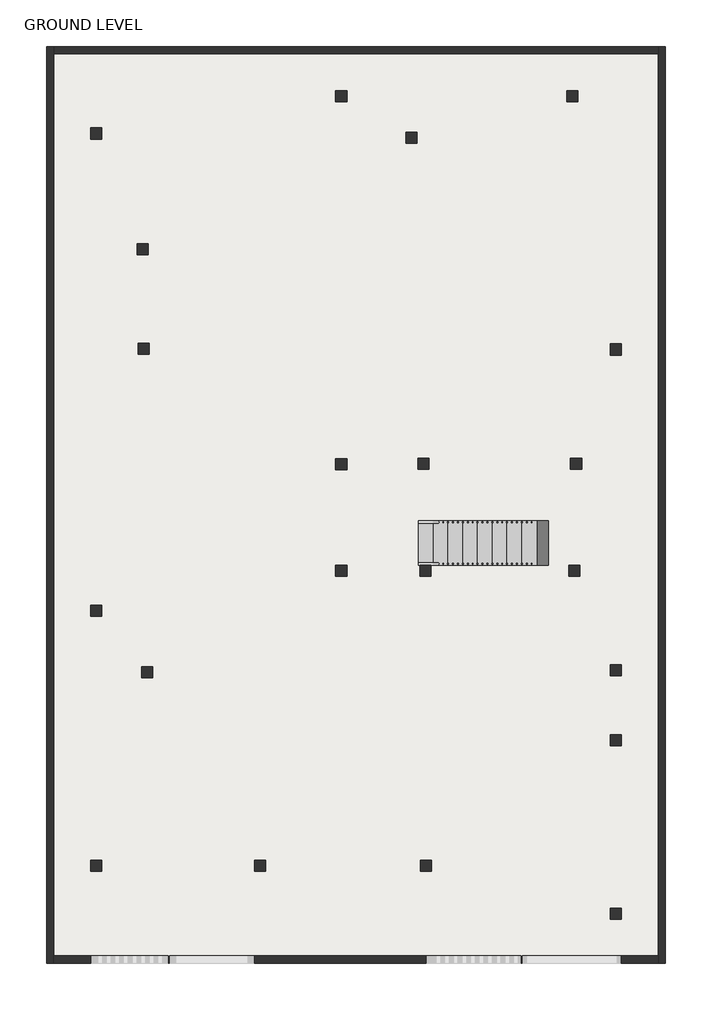
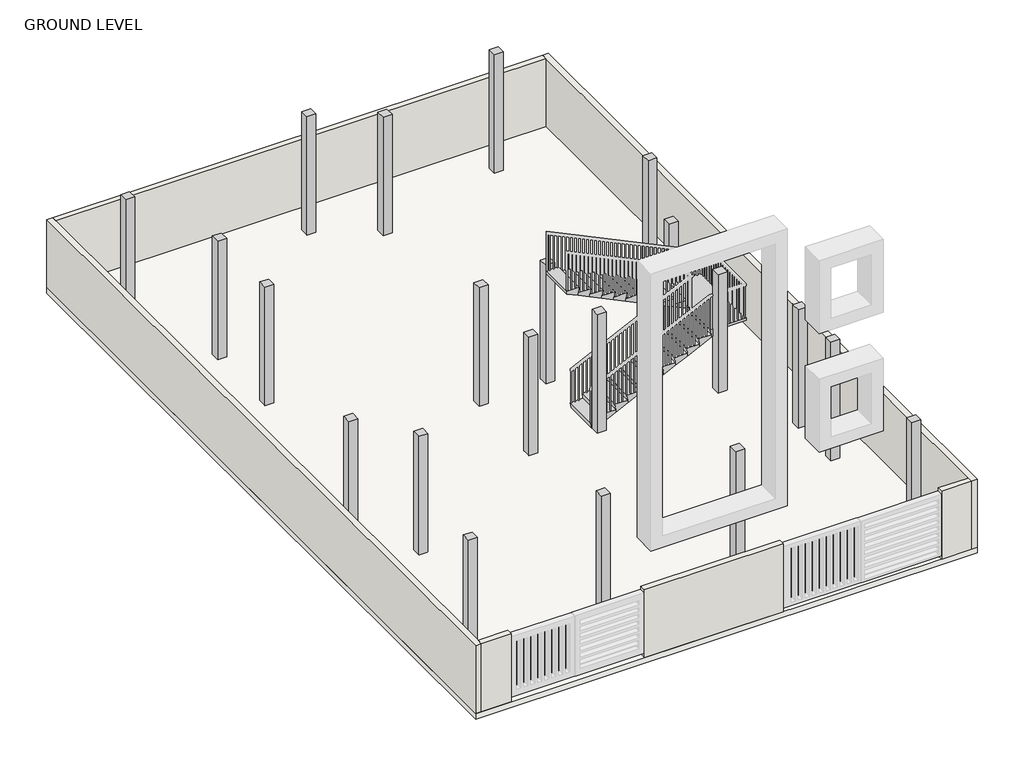
# One storey, part 1 of 3: 21 columns, 6 walls, 1 slab, 1 stair flight.
"""IFC4 building model written with IfcOpenShell, lengths in millimetres."""

from ifc_helpers import new_model, si_unit, frame, origin, origin_with_axes, place, context, project, spatial, polyline, outline, extrude, faceted_brep, element, save

model = new_model("IFC4")

# Units and contexts
model_context = context("Model", 3, world=origin())
ifc_project = project(units=[si_unit("LENGTHUNIT", "METRE", prefix="MILLI")], contexts=[model_context])

# Site, building, storey
site = spatial("IfcSite", under=ifc_project)
building = spatial("IfcBuilding", under=site)
storey = spatial("IfcBuildingStorey", under=building, Name="GROUND LEVEL", Elevation=0.0)

# Columns
placement = place(None, origin())
element("IfcColumn", 1, ObjectType="Rectangular Column : 9\"X9\"", at=placement, inside=storey, context=model_context, shape_type="SweptSolid", body=[
    extrude(outline(polyline([(-6539.8865981, 8531.2343988), (-6539.8865981, 8302.6343988), (-6768.4865981, 8302.6343988), (-6768.4865981, 8531.2343988), (-6539.8865981, 8531.2343988)])), origin_with_axes(), (0.0, 0.0, 1.0), 3200.4),
])
element("IfcColumn", 2, ObjectType="Rectangular Column : 9\"X9\"", at=placement, inside=storey, context=model_context, shape_type="SweptSolid", body=[
    extrude(outline(polyline([(-5558.0284021, 4080.4787587), (-5558.0284021, 3851.8787587), (-5786.6284021, 3851.8787587), (-5786.6284021, 4080.4787587), (-5558.0284021, 4080.4787587)])), origin_with_axes(), (0.0, 0.0, 1.0), 3200.4),
])
element("IfcColumn", 3, ObjectType="Rectangular Column : 9\"X9\"", at=placement, inside=storey, context=model_context, shape_type="SweptSolid", body=[
    extrude(outline(polyline([(-5488.7582398, -2599.7212413), (-5488.7582398, -2828.3212413), (-5717.3582398, -2828.3212413), (-5717.3582398, -2599.7212413), (-5488.7582398, -2599.7212413)])), origin_with_axes(), (0.0, 0.0, 1.0), 3200.4),
])
element("IfcColumn", 4, ObjectType="Rectangular Column : 9\"X9\"", at=placement, inside=storey, context=model_context, shape_type="SweptSolid", body=[
    extrude(outline(polyline([(-6539.8865981, -6601.1424416), (-6539.8865981, -6829.7424416), (-6768.4865981, -6829.7424416), (-6768.4865981, -6601.1424416), (-6539.8865981, -6601.1424416)])), origin_with_axes(), (0.0, 0.0, 1.0), 3200.4),
])
element("IfcColumn", 5, ObjectType="Rectangular Column : 9\"X9\"", at=placement, inside=storey, context=model_context, shape_type="SweptSolid", body=[
    extrude(outline(polyline([(-3148.9865981, -6600.2212413), (-3148.9865981, -6828.8212413), (-3377.5865981, -6828.8212413), (-3377.5865981, -6600.2212413), (-3148.9865981, -6600.2212413)])), origin_with_axes(), (0.0, 0.0, 1.0), 3200.4),
])
element("IfcColumn", 6, ObjectType="Rectangular Column : 9\"X9\"", at=placement, inside=storey, context=model_context, shape_type="SweptSolid", body=[
    extrude(outline(polyline([(280.0134019, -6601.1424416), (280.0134019, -6829.7424416), (51.4134019, -6829.7424416), (51.4134019, -6601.1424416), (280.0134019, -6601.1424416)])), origin_with_axes(), (0.0, 0.0, 1.0), 3200.4),
])
element("IfcColumn", 7, ObjectType="Rectangular Column : 9\"X9\"", at=placement, inside=storey, context=model_context, shape_type="SweptSolid", body=[
    extrude(outline(polyline([(4204.3134019, -7590.8212413), (4204.3134019, -7819.4212413), (3975.7134019, -7819.4212413), (3975.7134019, -7590.8212413), (4204.3134019, -7590.8212413)])), origin_with_axes(), (0.0, 0.0, 1.0), 3200.4),
])
element("IfcColumn", 8, ObjectType="Rectangular Column : 9\"X9\"", at=placement, inside=storey, context=model_context, shape_type="SweptSolid", body=[
    extrude(outline(polyline([(4204.3134019, -4009.4212413), (4204.3134019, -4238.0212413), (3975.7134019, -4238.0212413), (3975.7134019, -4009.4212413), (4204.3134019, -4009.4212413)])), origin_with_axes(), (0.0, 0.0, 1.0), 3200.4),
])
element("IfcColumn", 9, ObjectType="Rectangular Column : 9\"X9\"", at=placement, inside=storey, context=model_context, shape_type="SweptSolid", body=[
    extrude(outline(polyline([(3352.7127672, -504.2212413), (3352.7127672, -732.8212413), (3124.1127672, -732.8212413), (3124.1127672, -504.2212413), (3352.7127672, -504.2212413)])), origin_with_axes(), (0.0, 0.0, 1.0), 3200.4),
])
element("IfcColumn", 10, ObjectType="Rectangular Column : 9\"X9\"", at=placement, inside=storey, context=model_context, shape_type="SweptSolid", body=[
    extrude(outline(polyline([(269.7035962, -504.2212413), (269.7035962, -732.8212413), (41.1035962, -732.8212413), (41.1035962, -504.2212413), (269.7035962, -504.2212413)])), origin_with_axes(), (0.0, 0.0, 1.0), 3200.4),
])
element("IfcColumn", 11, ObjectType="Rectangular Column : 9\"X9\"", at=placement, inside=storey, context=model_context, shape_type="SweptSolid", body=[
    extrude(outline(polyline([(-1472.5865981, -505.1424416), (-1472.5865981, -733.7424416), (-1701.1865981, -733.7424416), (-1701.1865981, -505.1424416), (-1472.5865981, -505.1424416)])), origin_with_axes(), (0.0, 0.0, 1.0), 3200.4),
])
element("IfcColumn", 12, ObjectType="Rectangular Column : 9\"X9\"", at=placement, inside=storey, context=model_context, shape_type="SweptSolid", body=[
    extrude(outline(polyline([(-1472.5865981, 1693.0966521), (-1472.5865981, 1464.4966521), (-1701.1865981, 1464.4966521), (-1701.1865981, 1693.0966521), (-1472.5865981, 1693.0966521)])), origin_with_axes(), (0.0, 0.0, 1.0), 3200.4),
])
element("IfcColumn", 13, ObjectType="Rectangular Column : 9\"X9\"", at=placement, inside=storey, context=model_context, shape_type="SweptSolid", body=[
    extrude(outline(polyline([(229.251657, 1705.5787587), (229.251657, 1476.9787587), (0.651657, 1476.9787587), (0.651657, 1705.5787587), (229.251657, 1705.5787587)])), origin_with_axes(), (0.0, 0.0, 1.0), 3200.4),
])
element("IfcColumn", 14, ObjectType="Rectangular Column : 9\"X9\"", at=placement, inside=storey, context=model_context, shape_type="SweptSolid", body=[
    extrude(outline(polyline([(3385.1070369, 1705.5787587), (3385.1070369, 1476.9787587), (3156.5070369, 1476.9787587), (3156.5070369, 1705.5787587), (3385.1070369, 1705.5787587)])), origin_with_axes(), (0.0, 0.0, 1.0), 3200.4),
])
element("IfcColumn", 15, ObjectType="Rectangular Column : 9\"X9\"", at=placement, inside=storey, context=model_context, shape_type="SweptSolid", body=[
    extrude(outline(polyline([(4204.3134019, 4067.7787587), (4204.3134019, 3839.1787587), (3975.7134019, 3839.1787587), (3975.7134019, 4067.7787587), (4204.3134019, 4067.7787587)])), origin_with_axes(), (0.0, 0.0, 1.0), 3200.4),
])
element("IfcColumn", 16, ObjectType="Rectangular Column : 9\"X9\"", at=placement, inside=storey, context=model_context, shape_type="SweptSolid", body=[
    extrude(outline(polyline([(3305.8577655, 9300.1787587), (3305.8577655, 9071.5787587), (3077.2577655, 9071.5787587), (3077.2577655, 9300.1787587), (3305.8577655, 9300.1787587)])), origin_with_axes(), (0.0, 0.0, 1.0), 3200.4),
])
element("IfcColumn", 17, ObjectType="Rectangular Column : 9\"X9\"", at=placement, inside=storey, context=model_context, shape_type="SweptSolid", body=[
    extrude(outline(polyline([(-24.7865981, 8443.0921256), (-24.7865981, 8214.4921256), (-253.3865981, 8214.4921256), (-253.3865981, 8443.0921256), (-24.7865981, 8443.0921256)])), origin_with_axes(), (0.0, 0.0, 1.0), 3200.4),
])
element("IfcColumn", 18, ObjectType="Rectangular Column : 9\"X9\"", at=placement, inside=storey, context=model_context, shape_type="SweptSolid", body=[
    extrude(outline(polyline([(-5578.456564, 6137.8787587), (-5578.456564, 5909.2787587), (-5807.056564, 5909.2787587), (-5807.056564, 6137.8787587), (-5578.456564, 6137.8787587)])), origin_with_axes(), (0.0, 0.0, 1.0), 3200.4),
])
element("IfcColumn", 19, ObjectType="Rectangular Column : 9\"X9\"", at=placement, inside=storey, context=model_context, shape_type="SweptSolid", body=[
    extrude(outline(polyline([(-6539.8865981, -1329.7212413), (-6539.8865981, -1558.3212413), (-6768.4865981, -1558.3212413), (-6768.4865981, -1329.7212413), (-6539.8865981, -1329.7212413)])), origin_with_axes(), (0.0, 0.0, 1.0), 3200.4),
])
element("IfcColumn", 20, ObjectType="Rectangular Column : 9\"X9\"", at=placement, inside=storey, context=model_context, shape_type="SweptSolid", body=[
    extrude(outline(polyline([(4204.3134019, -2561.6212413), (4204.3134019, -2790.2212413), (3975.7134019, -2790.2212413), (3975.7134019, -2561.6212413), (4204.3134019, -2561.6212413)])), origin_with_axes(), (0.0, 0.0, 1.0), 3200.4),
])
element("IfcColumn", 21, ObjectType="Rectangular Column : 9\"X9\"", at=placement, inside=storey, context=model_context, shape_type="SweptSolid", body=[
    extrude(outline(polyline([(-1472.5865981, 9300.1787587), (-1472.5865981, 9071.5787587), (-1701.1865981, 9071.5787587), (-1701.1865981, 9300.1787587), (-1472.5865981, 9300.1787587)])), origin_with_axes(), (0.0, 0.0, 1.0), 3200.4),
])

# Slab
element("IfcSlab", 22, ObjectType="6\"", at=placement, inside=storey, context=model_context, shape_type="SweptSolid", body=[
    extrude(outline(polyline([(5118.7134019, 10214.5787587), (5118.7134019, -8733.8212413), (-7682.8865981, -8733.8212413), (-7682.8865981, 10214.5787587), (5118.7134019, 10214.5787587)])), frame((0.0, 0.0, -152.4), z_axis=(0.0, 0.0, 1.0), x_axis=(1.0, 0.0, 0.0)), (0.0, 0.0, 1.0), 152.4),
])

# Stair flight
element("IfcStairFlight", 23, ObjectType="3/4\" Nosing", at=placement, inside=storey, context=model_context, shape_type="Brep", body=[
    faceted_brep([(13.3134019, 410.1787587, 145.4727273), (13.3134019, -504.2212413, 145.4727273), (337.1634019, -504.2212413, 145.4727273), (337.1634019, 410.1787587, 145.4727273), (337.1634019, 410.1787587, 75.1111381), (179.7876839, 410.1787587, 0.0), (32.3634019, 410.1787587, 0.0), (32.3634019, -504.2212413, 0.0), (179.7876839, -504.2212413, 0.0), (337.1634019, -504.2212413, 75.1111381), (318.1134019, 410.1787587, 290.9454545), (318.1134019, -504.2212413, 290.9454545), (641.9634019, -504.2212413, 290.9454545), (641.9634019, 410.1787587, 290.9454545), (641.9634019, 410.1787587, 220.5838654), (641.9634019, -504.2212413, 220.5838654), (622.9134019, 410.1787587, 436.4181818), (622.9134019, -504.2212413, 436.4181818), (946.7634019, -504.2212413, 436.4181818), (946.7634019, 410.1787587, 436.4181818), (946.7634019, 410.1787587, 366.0565927), (946.7634019, -504.2212413, 366.0565927), (927.7134019, 410.1787587, 581.8909091), (927.7134019, -504.2212413, 581.8909091), (1251.5634019, -504.2212413, 581.8909091), (1251.5634019, 410.1787587, 581.8909091), (1251.5634019, 410.1787587, 511.5293199), (1251.5634019, -504.2212413, 511.5293199), (1232.5134019, 410.1787587, 727.3636364), (1232.5134019, -504.2212413, 727.3636364), (1556.3634019, -504.2212413, 727.3636364), (1556.3634019, 410.1787587, 727.3636364), (1556.3634019, 410.1787587, 657.0020472), (1556.3634019, -504.2212413, 657.0020472), (1537.3134019, 410.1787587, 872.8363636), (1537.3134019, -504.2212413, 872.8363636), (1861.1634019, -504.2212413, 872.8363636), (1861.1634019, 410.1787587, 872.8363636), (1861.1634019, 410.1787587, 802.4747745), (1861.1634019, -504.2212413, 802.4747745), (1842.1134019, 410.1787587, 1018.3090909), (1842.1134019, -504.2212413, 1018.3090909), (2165.9634019, -504.2212413, 1018.3090909), (2165.9634019, 410.1787587, 1018.3090909), (2165.9634019, 410.1787587, 947.9475018), (2165.9634019, -504.2212413, 947.9475018), (2146.9134019, 410.1787587, 1163.7818182), (2146.9134019, -504.2212413, 1163.7818182), (2470.7634019, -504.2212413, 1163.7818182), (2470.7634019, 410.1787587, 1163.7818182), (2470.7634019, 410.1787587, 1093.420229), (2470.7634019, -504.2212413, 1093.420229), (2451.7134019, 410.1787587, 1309.2545455), (2451.7134019, -504.2212413, 1309.2545455), (2775.5634019, -504.2212413, 1309.2545455), (2775.5634019, 410.1787587, 1309.2545455), (2775.5634019, 410.1787587, 1238.8929563), (2775.5634019, -504.2212413, 1238.8929563), (3080.3634019, 410.1787587, 1454.7272727), (2756.5134019, 410.1787587, 1454.7272727), (2756.5134019, -504.2212413, 1454.7272727), (3080.3634019, -504.2212413, 1454.7272727), (3069.628878, 410.1787587, 1536.7), (3399.5400648, 410.1787587, 1536.7), (3080.3634019, -504.2212413, 1384.3656836), (3042.2634019, 562.5787587, 1600.2), (3061.3134019, 562.5787587, 1600.2), (3061.3134019, 410.1787587, 1600.2), (3061.3134019, -504.2212413, 1600.2), (3399.5400648, -504.2212413, 1600.2), (3975.7134019, -504.2212413, 1600.2), (3975.7134019, 1476.9787587, 1600.2), (3042.2634019, 1476.9787587, 1600.2), (3042.2634019, 562.5787587, 1536.7), (3061.3134019, 562.5787587, 1536.7), (3061.3134019, 410.1787587, 1536.7), (3399.5400648, -504.2212413, 1536.7), (3975.7134019, -504.2212413, 1536.7), (3975.7134019, 1476.9787587, 1536.7), (3042.2634019, 1476.9787587, 1536.7), (3061.3134019, 562.5787587, 1745.6727273), (3061.3134019, 1476.9787587, 1745.6727273), (3027.8867389, 1476.9787587, 1745.6727273), (2737.4634019, 1476.9787587, 1745.6727273), (2737.4634019, 562.5787587, 1745.6727273), (3027.8867389, 562.5787587, 1745.6727273), (2737.4634019, 562.5787587, 1675.3111381), (3027.8867389, 562.5787587, 1536.7), (3027.8867389, 1476.9787587, 1536.7), (2737.4634019, 1476.9787587, 1675.3111381), (2756.5134019, 562.5787587, 1891.1454545), (2756.5134019, 1476.9787587, 1891.1454545), (2432.6634019, 1476.9787587, 1891.1454545), (2432.6634019, 562.5787587, 1891.1454545), (2432.6634019, 562.5787587, 1820.7838654), (2432.6634019, 1476.9787587, 1820.7838654), (2451.7134019, 562.5787587, 2036.6181818), (2451.7134019, 1476.9787587, 2036.6181818), (2127.8634019, 1476.9787587, 2036.6181818), (2127.8634019, 562.5787587, 2036.6181818), (2127.8634019, 562.5787587, 1966.2565927), (2127.8634019, 1476.9787587, 1966.2565927), (2146.9134019, 562.5787587, 2182.0909091), (2146.9134019, 1476.9787587, 2182.0909091), (1823.0634019, 1476.9787587, 2182.0909091), (1823.0634019, 562.5787587, 2182.0909091), (1823.0634019, 562.5787587, 2111.7293199), (1823.0634019, 1476.9787587, 2111.7293199), (1842.1134019, 562.5787587, 2327.5636364), (1842.1134019, 1476.9787587, 2327.5636364), (1518.2634019, 1476.9787587, 2327.5636364), (1518.2634019, 562.5787587, 2327.5636364), (1518.2634019, 562.5787587, 2257.2020472), (1518.2634019, 1476.9787587, 2257.2020472), (1537.3134019, 562.5787587, 2473.0363636), (1537.3134019, 1476.9787587, 2473.0363636), (1213.4634019, 1476.9787587, 2473.0363636), (1213.4634019, 562.5787587, 2473.0363636), (1213.4634019, 562.5787587, 2402.6747745), (1213.4634019, 1476.9787587, 2402.6747745), (1232.5134019, 562.5787587, 2618.5090909), (1232.5134019, 1476.9787587, 2618.5090909), (908.6634019, 1476.9787587, 2618.5090909), (908.6634019, 562.5787587, 2618.5090909), (908.6634019, 562.5787587, 2548.1475018), (908.6634019, 1476.9787587, 2548.1475018), (927.7134019, 562.5787587, 2763.9818182), (927.7134019, 1476.9787587, 2763.9818182), (603.8634019, 1476.9787587, 2763.9818182), (603.8634019, 562.5787587, 2763.9818182), (603.8634019, 562.5787587, 2693.620229), (603.8634019, 1476.9787587, 2693.620229), (622.9134019, 562.5787587, 2909.4545455), (622.9134019, 1476.9787587, 2909.4545455), (299.0634019, 1476.9787587, 2909.4545455), (299.0634019, 562.5787587, 2909.4545455), (299.0634019, 562.5787587, 2839.0929563), (299.0634019, 1476.9787587, 2839.0929563), (318.1134019, 562.5787587, 3054.9272727), (318.1134019, 1476.9787587, 3054.9272727), (13.3134019, 1476.9787587, 3054.9272727), (13.3134019, 562.5787587, 3054.9272727), (13.3134019, 562.5787587, 2975.4736381), (13.3134019, 1476.9787587, 2975.4736381)], [[[0, 1, 2, 3]], [[0, 3, 4, 5, 6]], [[2, 1, 7, 8, 9]], [[10, 11, 12, 13]], [[10, 13, 14, 4, 3]], [[12, 11, 2, 9, 15]], [[16, 17, 18, 19]], [[16, 19, 20, 14, 13]], [[18, 17, 12, 15, 21]], [[22, 23, 24, 25]], [[22, 25, 26, 20, 19]], [[24, 23, 18, 21, 27]], [[28, 29, 30, 31]], [[28, 31, 32, 26, 25]], [[30, 29, 24, 27, 33]], [[34, 35, 36, 37]], [[34, 37, 38, 32, 31]], [[36, 35, 30, 33, 39]], [[40, 41, 42, 43]], [[40, 43, 44, 38, 37]], [[42, 41, 36, 39, 45]], [[46, 47, 48, 49]], [[46, 49, 50, 44, 43]], [[48, 47, 42, 45, 51]], [[52, 53, 54, 55]], [[52, 55, 56, 50, 49]], [[54, 53, 48, 51, 57]], [[58, 59, 60, 61]], [[58, 62, 63, 56, 55, 59]], [[61, 60, 54, 57, 64]], [[65, 66, 67, 68, 69, 70, 71, 72]], [[66, 65, 73, 74]], [[67, 66, 74, 75]], [[62, 67, 75]], [[68, 61, 64, 76, 77, 70, 69]], [[71, 70, 77, 78]], [[72, 71, 78, 79]], [[80, 81, 82, 83, 84, 85]], [[65, 80, 85, 84, 86, 87, 73]], [[81, 72, 79, 88, 89, 83, 82]], [[90, 91, 92, 93]], [[90, 93, 94, 86, 84]], [[92, 91, 83, 89, 95]], [[96, 97, 98, 99]], [[96, 99, 100, 94, 93]], [[98, 97, 92, 95, 101]], [[102, 103, 104, 105]], [[102, 105, 106, 100, 99]], [[104, 103, 98, 101, 107]], [[108, 109, 110, 111]], [[108, 111, 112, 106, 105]], [[110, 109, 104, 107, 113]], [[114, 115, 116, 117]], [[114, 117, 118, 112, 111]], [[116, 115, 110, 113, 119]], [[120, 121, 122, 123]], [[120, 123, 124, 118, 117]], [[122, 121, 116, 119, 125]], [[126, 127, 128, 129]], [[126, 129, 130, 124, 123]], [[128, 127, 122, 125, 131]], [[132, 133, 134, 135]], [[132, 135, 136, 130, 129]], [[134, 133, 128, 131, 137]], [[1, 0, 6, 7]], [[3, 2, 11, 10]], [[13, 12, 17, 16]], [[19, 18, 23, 22]], [[25, 24, 29, 28]], [[31, 30, 35, 34]], [[37, 36, 41, 40]], [[43, 42, 47, 46]], [[49, 48, 53, 52]], [[55, 54, 60, 59]], [[58, 61, 68, 67, 62]], [[65, 72, 81, 80]], [[84, 83, 91, 90]], [[93, 92, 97, 96]], [[99, 98, 103, 102]], [[105, 104, 109, 108]], [[111, 110, 115, 114]], [[117, 116, 121, 120]], [[123, 122, 127, 126]], [[129, 128, 133, 132]], [[138, 139, 140, 141]], [[138, 141, 142, 136, 135]], [[140, 139, 134, 137, 143]], [[141, 140, 143, 142]], [[135, 134, 139, 138]], [[7, 6, 5, 8]], [[56, 63, 76, 64, 57, 51, 45, 39, 33, 27, 21, 15, 9, 8, 5, 4, 14, 20, 26, 32, 38, 44, 50]], [[76, 63, 62, 75, 74, 73, 87, 88, 79, 78, 77]], [[88, 87, 86, 94, 100, 106, 112, 118, 124, 130, 136, 142, 143, 137, 131, 125, 119, 113, 107, 101, 95, 89]]]),
])

# Walls
element("IfcWall", 24, ObjectType="6\"", at=placement, inside=storey, context=model_context, shape_type="Brep", body=[
    faceted_brep([(-7682.8865981, 10214.5787587, 0.0), (-7682.8865981, -8733.8212413, 0.0), (-7682.8865981, -8733.8212413, 1828.8), (-7682.8865981, 10214.5787587, 1828.8), (-7530.4865981, 10214.5787587, 0.0), (-7530.4865981, 10214.5787587, 1828.8), (-7530.4865981, 10062.1787587, 1828.8), (-7530.4865981, -8581.4212413, 1828.8), (-7530.4865981, -8733.8212413, 1828.8), (-7530.4865981, -8733.8212413, 0.0), (-7530.4865981, -8581.4212413, 0.0), (-7530.4865981, 10062.1787587, 0.0)], [[[0, 1, 2, 3]], [[4, 5, 6, 7, 8, 9, 10, 11]], [[1, 0, 4, 11, 10, 9]], [[3, 2, 8, 7, 6, 5]], [[2, 1, 9, 8]], [[0, 3, 5, 4]]]),
])
element("IfcWall", 25, ObjectType="6\"", at=placement, inside=storey, context=model_context, shape_type="SweptSolid", body=[
    extrude(outline(polyline([(-6768.4865981, -8733.8212413), (-7530.4865981, -8733.8212413), (-7530.4865981, -8581.4212413), (-6768.4865981, -8581.4212413), (-6768.4865981, -8733.8212413)])), origin_with_axes(), (0.0, 0.0, 1.0), 1828.8),
])
element("IfcWall", 26, ObjectType="6\"", at=placement, inside=storey, context=model_context, shape_type="Brep", body=[
    faceted_brep([(4966.3134019, 10214.5787587, 0.0), (4966.3134019, 10062.1787587, 0.0), (4966.3134019, -8581.4212413, 0.0), (4966.3134019, -8733.8212413, 0.0), (4966.3134019, -8733.8212413, 1828.8), (4966.3134019, -8581.4212413, 1828.8), (4966.3134019, 10062.1787587, 1828.8), (4966.3134019, 10214.5787587, 1828.8), (5118.7134019, 10214.5787587, 0.0), (5118.7134019, 10214.5787587, 1828.8), (5118.7134019, -8733.8212413, 1828.8), (5118.7134019, -8733.8212413, 0.0)], [[[0, 1, 2, 3, 4, 5, 6, 7]], [[8, 9, 10, 11]], [[3, 2, 1, 0, 8, 11]], [[7, 6, 5, 4, 10, 9]], [[4, 3, 11, 10]], [[0, 7, 9, 8]]]),
])
element("IfcWall", 27, ObjectType="6\"", at=placement, inside=storey, context=model_context, shape_type="SweptSolid", body=[
    extrude(outline(polyline([(4204.3134019, -8581.4212413), (4966.3134019, -8581.4212413), (4966.3134019, -8733.8212413), (4204.3134019, -8733.8212413), (4204.3134019, -8581.4212413)])), origin_with_axes(), (0.0, 0.0, 1.0), 1828.8),
])
element("IfcWall", 28, ObjectType="6\"", at=placement, inside=storey, context=model_context, shape_type="SweptSolid", body=[
    extrude(outline(polyline([(-3377.5865981, -8581.4212413), (165.7134019, -8581.4212413), (165.7134019, -8733.8212413), (-3377.5865981, -8733.8212413), (-3377.5865981, -8581.4212413)])), origin_with_axes(), (0.0, 0.0, 1.0), 1828.8),
])
element("IfcWall", 29, ObjectType="6\"", at=placement, inside=storey, context=model_context, shape_type="SweptSolid", body=[
    extrude(outline(polyline([(-7530.4865981, 10214.5787587), (4966.3134019, 10214.5787587), (4966.3134019, 10062.1787587), (-7530.4865981, 10062.1787587), (-7530.4865981, 10214.5787587)])), origin_with_axes(), (0.0, 0.0, 1.0), 1828.8),
])

save(model, "model.ifc")

# Revit data of these elements
# Type "Rectangular Column : 9\"X9\""
#   Assembly Code = "B1010200"
#   Depth = 0' - 9"
#   Offset Base = 0' - 0"
#   Offset Top = 0' - 0"
#   Width = 0' - 9"
#   Material = none
# Type "6\""
#   Assembly Code = "B1010"
#   Function = 0
#   Layers, outside or top first: 0' - 6" no material (function 1)
# Type "6\""
#   Assembly Code = "B2010"
#   Layers, outside or top first: 0' - 6" "wood 1" (function 1)
# Elements 1, 2, 3, 4, 5, 6, 7, 8, 9, 10, 11, 12, 13, 14, 15, 16, 17, 18, 19, 20, 21 (IfcColumn, "Rectangular Column : 9\"X9\"")
#   Phase Created = New Construction
# Element 22 (IfcSlab, "6\"")
#   Height Offset From Level = 0' - 0"
#   Phase Created = New Construction
#   Materials on its faces: "Default Floor"
# Element 23 (IfcStairFlight, "3/4\" Nosing")
#   Phase Created = New Construction
#   Materials on its faces: "Concrete, Cast-in-Place gray"
# Elements 24, 25, 26, 27, 28, 29 (IfcWall, "6\"")
#   Top Offset = 0' - 0"
#   Base Offset = 0' - 0"
#   Unconnected Height = 6' - 0"
#   wall height = 6' - 0"
#   Phase Created = New Construction
#   Base Constraint = GROUND LEVEL
#   Materials on its faces: "wood 1"
# Materials
#   "wood 1": class "Generic", colour RGB 88 94 108, transparency 0, Cost = 0
#   "Default Floor": colour RGB 128 128 128, transparency 0, Cost = 0
#   "Concrete, Cast-in-Place gray": class "Concrete", colour RGB 192 192 192, transparency 0, Description = "Cast-in-place concrete", Cost = 0
